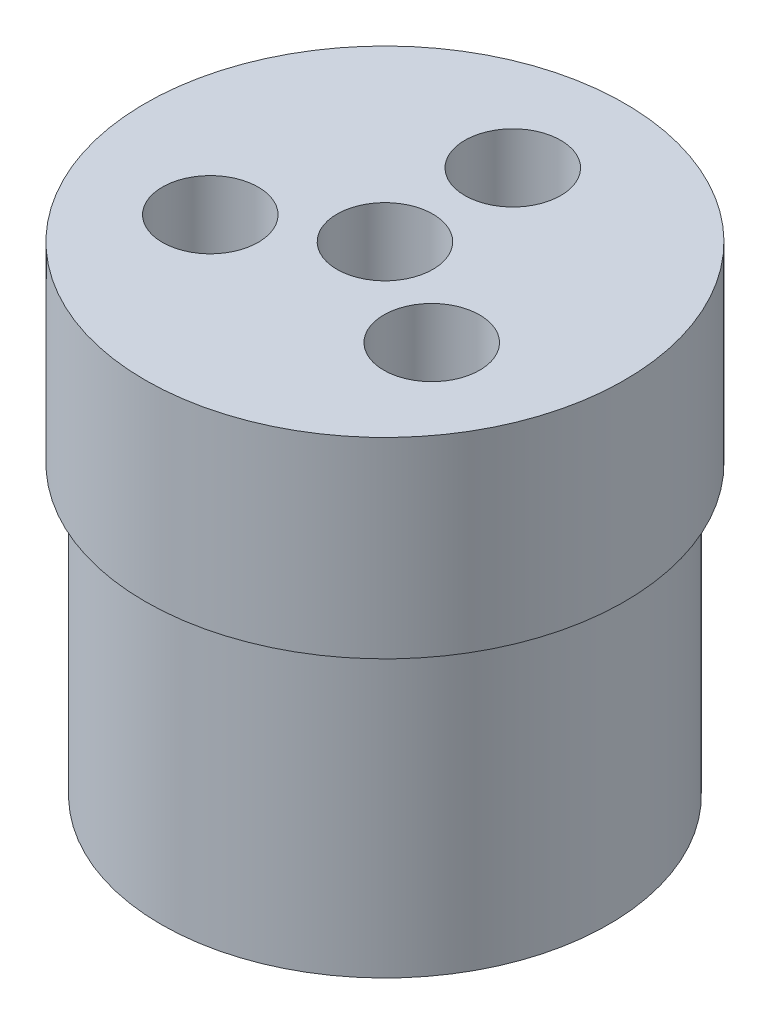
from build123d import *

# Parameters (mm, degrees)
UPPER_BODY_PROFILE_30_R         = 15
UPPER_BODY_30X12_DEPTH          = 12
LOWER_BODY_PROFILE_28_R         = 14
LOWER_BODY_28X18_DEPTH          = 18
OFFSET_HOLES_PROFILE_3X_6_R     = 3
OFFSET_THROUGH_HOLES_3X_6_DEPTH = 44
CENTER_HOLE_PROFILE_6_R         = 3
CENTER_THROUGH_HOLE_6_DEPTH     = 44


with BuildPart() as part:
    # Upper Body Profile Ø30 → Upper Body Ø30x12 (new body)
    with BuildSketch(Plane(origin=(0, 0, 0), x_dir=(1, 0, 0), z_dir=(0, 1, 0))):
        with Locations(Location((0, 0, 0), (0, 0, 270))):
            Circle(UPPER_BODY_PROFILE_30_R)
    extrude(amount=UPPER_BODY_30X12_DEPTH)

    # Lower Body Profile Ø28 → Lower Body Ø28x18 (add)
    with BuildSketch(Plane.XZ):
        with Locations(Location((0, 0, 0), (0, 0, 270))):
            Circle(LOWER_BODY_PROFILE_28_R)
    extrude(amount=LOWER_BODY_28X18_DEPTH)

    # Offset Holes Profile 3xØ6 → Offset Through Holes 3xØ6 (cut)
    with BuildSketch(Plane(origin=(0, 12, 0), x_dir=(1, 0, 0), z_dir=(0, 1, 0))):
        with Locations(Location((0, 8, 0), (0, 0, 270))):
            Circle(OFFSET_HOLES_PROFILE_3X_6_R)
        with Locations(Location((6.92820323, -4, 0), (0, 0, 270))):
            Circle(OFFSET_HOLES_PROFILE_3X_6_R)
        with Locations(Location((-6.92820323, -4, 0), (0, 0, 270))):
            Circle(OFFSET_HOLES_PROFILE_3X_6_R)
    extrude(amount=-OFFSET_THROUGH_HOLES_3X_6_DEPTH, mode=Mode.SUBTRACT)

    # Center Hole Profile Ø6 → Center Through Hole Ø6 (cut)
    with BuildSketch(Plane(origin=(0, 12, 0), x_dir=(1, 0, 0), z_dir=(0, 1, 0))):
        with Locations(Location((0, 0, 0), (0, 0, 270))):
            Circle(CENTER_HOLE_PROFILE_6_R)
    extrude(amount=-CENTER_THROUGH_HOLE_6_DEPTH, mode=Mode.SUBTRACT)


solid = part.part
